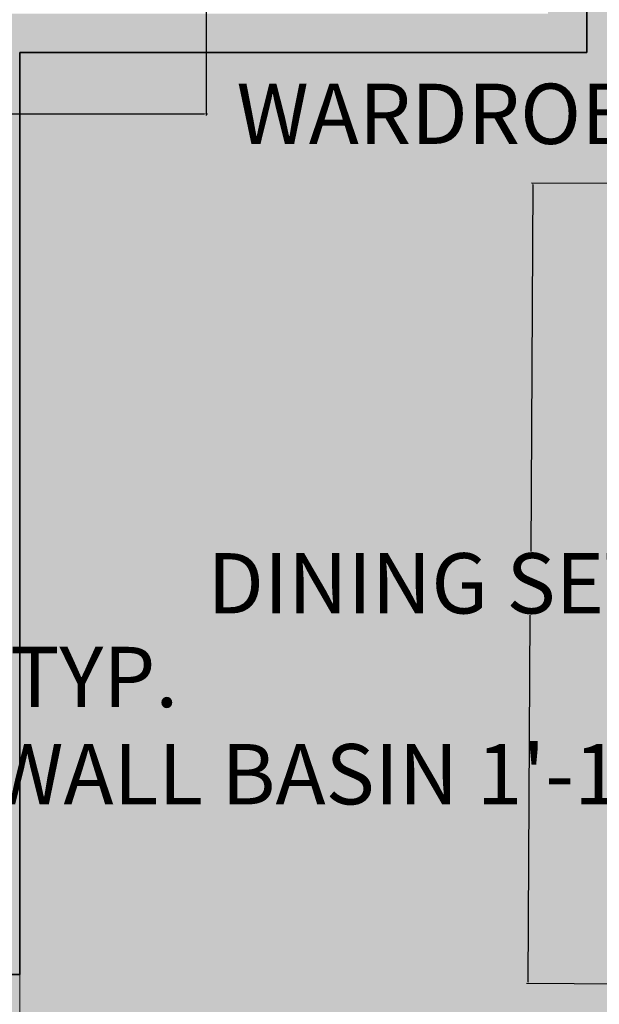
# Model space of a CAD drawing. Units: inches. Extents: x 1316 to 1777, y 813 to 1650.
# Tile 8 of 22: x 1445 to 1512, y 1319 to 1434. Entities that reach past the tile are written whole.
import ezdxf

# ---------------------------------------------------------------- set-up
doc = ezdxf.new("R2010")
doc.units = ezdxf.units.IN
doc.header["$MEASUREMENT"] = 0
doc.linetypes.add('ACAD_ISO02W100', pattern=[15, 12, -3])
for name, color, linetype, lineweight in [('A-ANNO-DIMS', 2, 'Continuous', 18), ('A-WALL-OVHD', 250, 'ACAD_ISO02W100', 18), ('A-WALL-PATT', 250, 'Continuous', 13), ('walls', 250, 'Continuous', 35)]:
    doc.layers.add(name, color=color, linetype=linetype, lineweight=lineweight)
doc.layers.add('A-FLOR-PATT', color=254, linetype='Continuous', lineweight=13, true_color=0xfeeab9)
doc.styles.get("Standard").update_dxf_attribs({"font": 'arial.ttf'})
doc.dimstyles.get("Standard").update_dxf_attribs({"dimtxt": 7, "dimasz": 0.18, "dimexe": 0.18, "dimexo": 0.0625, "dimgap": 0.09, "dimtad": 0, "dimtih": 1, "dimtoh": 1, "dimzin": 0, "dimdsep": 46, "dimlunit": 3, "dimtxsty": 'Standard', "dimcen": 0.09, "dimadec": 0, "dimazin": 0, "dimtfac": 1, "dimtofl": 0, "dimtmove": 0, "dimatfit": 3, "dimfxl": 1, "dimtolj": 1, "dimtzin": 0, "dimarcsym": 0})

# ---------------------------------------------------------------- blocks, each defined once
blk = doc.blocks.new('*D30')
at = {"layer": 'A-ANNO-DIMS', "color": 0, "lineweight": -2, "transparency": 16777216}
for p, q in [((1386.15, 1434.7), (1386.15, 1422.58)), ((1466.18, 1434.7), (1466.18, 1422.58)), ((1386.33, 1422.76), (1466, 1422.76)), ((1466.18, 1422.76), (1466.36, 1422.76))]:
    blk.add_line(p, q, dxfattribs=at)
at = {"layer": 'A-ANNO-DIMS', "color": 0, "transparency": 16777216}
for points in [[(1386.33, 1422.79), (1386.33, 1422.73), (1386.15, 1422.76)], [(1466, 1422.79), (1466, 1422.73), (1466.18, 1422.76)]]:
    blk.add_solid(points, dxfattribs=at)
at = {"layer": 'Defpoints', "color": 0, "transparency": 16777216}
for p in [(1386.15, 1434.76), (1466.18, 1434.76), (1466.18, 1422.76)]:
    blk.add_point(p, dxfattribs=at)
at = {"layer": 'A-ANNO-DIMS', "color": 0, "transparency": 16777216, "insert": (1518.08, 1422.76), "char_height": 7, "attachment_point": 5}
blk.add_mtext('\\A1;WARDROBE 6\'-8" TYP.', dxfattribs=at)
blk = doc.blocks.new('*D31')
at = {"layer": 'A-ANNO-DIMS', "color": 0, "lineweight": -2, "transparency": 16777216}
for p, q in [((1466.24, 1450.33), (1478.36, 1450.33)), ((1478.18, 1450.15), (1478.18, 1446.26)), ((1478.18, 1434.94), (1478.18, 1438.83)), ((1466.24, 1434.76), (1478.36, 1434.76))]:
    blk.add_line(p, q, dxfattribs=at)
at = {"layer": 'A-ANNO-DIMS', "color": 0, "transparency": 16777216}
for points in [[(1478.15, 1450.15), (1478.21, 1450.15), (1478.18, 1450.33)], [(1478.15, 1434.94), (1478.21, 1434.94), (1478.18, 1434.76)]]:
    blk.add_solid(points, dxfattribs=at)
at = {"layer": 'Defpoints', "color": 0, "transparency": 16777216}
for p in [(1466.18, 1450.33), (1478.18, 1450.33), (1466.18, 1434.76)]:
    blk.add_point(p, dxfattribs=at)
at = {"layer": 'A-ANNO-DIMS', "color": 0, "transparency": 16777216, "insert": (1478.18, 1442.55), "char_height": 7, "attachment_point": 5}
blk.add_mtext('\\A1;1\'-3 1/2" TYP.', dxfattribs=at)
blk = doc.blocks.new('*D36')
at = {"layer": 'A-ANNO-DIMS', "color": 0, "lineweight": -2, "transparency": 16777216}
for p, q in [((1416.11, 1349.39), (1416.11, 1345.95)), ((1438.26, 1349.39), (1438.26, 1345.95)), ((1416.29, 1346.13), (1438.08, 1346.13)), ((1438.26, 1346.13), (1438.44, 1346.13))]:
    blk.add_line(p, q, dxfattribs=at)
at = {"layer": 'A-ANNO-DIMS', "color": 0, "transparency": 16777216}
for points in [[(1416.29, 1346.16), (1416.29, 1346.1), (1416.11, 1346.13)], [(1438.08, 1346.16), (1438.08, 1346.1), (1438.26, 1346.13)]]:
    blk.add_solid(points, dxfattribs=at)
at = {"layer": 'Defpoints', "color": 0, "transparency": 16777216}
for p in [(1416.11, 1349.46), (1438.26, 1349.46), (1438.26, 1346.13)]:
    blk.add_point(p, dxfattribs=at)
at = {"layer": 'A-ANNO-DIMS', "color": 0, "transparency": 16777216, "insert": (1493.43, 1346.13), "char_height": 7, "attachment_point": 5}
blk.add_mtext('\\A1;WALL BASIN 1\'-10" TYP.', dxfattribs=at)
blk = doc.blocks.new('*D37')
at = {"layer": 'A-ANNO-DIMS', "color": 0, "lineweight": -2, "transparency": 16777216}
for p, q in [((1438.33, 1365.37), (1441.77, 1365.37)), ((1441.59, 1365.19), (1441.59, 1361.02)), ((1441.59, 1349.64), (1441.59, 1353.81)), ((1438.33, 1349.46), (1441.77, 1349.46))]:
    blk.add_line(p, q, dxfattribs=at)
at = {"layer": 'A-ANNO-DIMS', "color": 0, "transparency": 16777216}
for points in [[(1441.56, 1365.19), (1441.62, 1365.19), (1441.59, 1365.37)], [(1441.56, 1349.64), (1441.62, 1349.64), (1441.59, 1349.46)]]:
    blk.add_solid(points, dxfattribs=at)
at = {"layer": 'Defpoints', "color": 0, "transparency": 16777216}
for p in [(1438.26, 1365.37), (1441.59, 1365.37), (1438.26, 1349.46)]:
    blk.add_point(p, dxfattribs=at)
at = {"layer": 'A-ANNO-DIMS', "color": 0, "transparency": 16777216, "insert": (1441.59, 1357.41), "char_height": 7, "attachment_point": 5}
blk.add_mtext('\\A1;1\'-4" TYP.', dxfattribs=at)
blk = doc.blocks.new('*D40')
at = {"layer": 'A-ANNO-DIMS', "color": 0, "lineweight": -2, "transparency": 16777216}
for p, q in [((1388.84, 1302.16), (1388.84, 1312.14)), ((1389.02, 1311.96), (1454.4, 1311.96)), ((1454.58, 1302.16), (1454.58, 1312.14)), ((1454.58, 1311.96), (1454.76, 1311.96))]:
    blk.add_line(p, q, dxfattribs=at)
at = {"layer": 'A-ANNO-DIMS', "color": 0, "transparency": 16777216}
for points in [[(1389.02, 1311.99), (1389.02, 1311.93), (1388.84, 1311.96)], [(1454.4, 1311.99), (1454.4, 1311.93), (1454.58, 1311.96)]]:
    blk.add_solid(points, dxfattribs=at)
at = {"layer": 'Defpoints', "color": 0, "transparency": 16777216}
for p in [(1454.58, 1311.96), (1388.84, 1302.1), (1454.58, 1302.1)]:
    blk.add_point(p, dxfattribs=at)
at = {"layer": 'A-ANNO-DIMS', "color": 0, "transparency": 16777216, "insert": (1507.74, 1311.96), "char_height": 7, "attachment_point": 5}
blk.add_mtext('\\A1;KITCHEN SINK 5\'-5 1/2"', dxfattribs=at)
blk = doc.blocks.new('*D42')
at = {"layer": 'A-ANNO-DIMS', "color": 0, "lineweight": -2, "transparency": 16777216}
for p, q in [((1388.61, 1310.85), (1388.61, 1307.49)), ((1410.21, 1310.85), (1410.21, 1307.49)), ((1388.79, 1307.67), (1410.03, 1307.67)), ((1410.21, 1307.67), (1410.39, 1307.67))]:
    blk.add_line(p, q, dxfattribs=at)
at = {"layer": 'A-ANNO-DIMS', "color": 0, "transparency": 16777216}
for points in [[(1388.79, 1307.7), (1388.79, 1307.64), (1388.61, 1307.67)], [(1410.03, 1307.7), (1410.03, 1307.64), (1410.21, 1307.67)]]:
    blk.add_solid(points, dxfattribs=at)
at = {"layer": 'Defpoints', "color": 0, "transparency": 16777216}
for p in [(1388.61, 1310.91), (1410.21, 1310.91), (1410.21, 1307.67)]:
    blk.add_point(p, dxfattribs=at)
at = {"layer": 'A-ANNO-DIMS', "color": 0, "transparency": 16777216, "insert": (1453.71, 1307.67), "char_height": 7, "attachment_point": 5}
blk.add_mtext('\\A1;COOKTOP 1\'-9 1/2"', dxfattribs=at)
blk = doc.blocks.new('*D48')
at = {"layer": 'A-ANNO-DIMS', "color": 0, "lineweight": -2, "transparency": 16777216}
for p, q in [((1504.09, 1414.55), (1503.83, 1371.99)), ((1517.96, 1414.64), (1503.91, 1414.73)), ((1503.52, 1322.01), (1503.78, 1364.57)), ((1517.39, 1321.74), (1503.34, 1321.83))]:
    blk.add_line(p, q, dxfattribs=at)
at = {"layer": 'A-ANNO-DIMS', "color": 0, "transparency": 16777216}
for points in [[(1504.06, 1414.55), (1504.12, 1414.55), (1504.09, 1414.73)], [(1503.49, 1322.01), (1503.55, 1322.01), (1503.52, 1321.83)]]:
    blk.add_solid(points, dxfattribs=at)
at = {"layer": 'Defpoints', "color": 0, "transparency": 16777216}
for p in [(1518.02, 1414.64), (1503.52, 1321.83), (1517.46, 1321.74)]:
    blk.add_point(p, dxfattribs=at)
at = {"layer": 'A-ANNO-DIMS', "color": 0, "transparency": 16777216, "insert": (1503.81, 1368.28), "char_height": 7, "attachment_point": 5}
blk.add_mtext('\\A1;DINING SET 7\'-9"', dxfattribs=at)

msp = doc.modelspace()

# ---------------------------------------------------------------- hatches: boundary and pattern name
at = {"layer": 'A-FLOR-PATT'}
h = msp.add_hatch(color=256, dxfattribs=at)
h.dxf.hatch_style = 1
h.paths.add_polyline_path([(1567.673, 1281.369), (1651.673, 1281.369), (1651.673, 1365.369), (1597.673, 1365.369), (1597.673, 1429.869), (1570.345, 1429.869), (1570.345, 1471.869), (1510.345, 1471.869), (1510.345, 1429.869), (1444.564, 1429.869), (1444.564, 1322.882), (1444.564, 1300.088), (1510.564, 1300.088), (1510.564, 1295.094), (1510.564, 1240.869), (1386.064, 1240.869), (1386.064, 1171.185), (1400.961, 1171.185), (1400.961, 1106.742), (1386.064, 1106.742), (1386.064, 1072.869), (1510.564, 1072.869), (1510.564, 1040.173), (1541.068, 1040.173, -0.367085), (1572.764, 1069.547), (1572.764, 1069.579), (1574.225, 1069.579), (1574.225, 1040.173), (1616.037, 1040.173), (1616.037, 1086.627), (1616.037, 1103.705), (1613.066, 1105.235), (1616.037, 1106.686), (1616.037, 1123.869), (1567.673, 1123.869)])
h.paths.add_polyline_path([(1508.987, 1198.018), (1511.117, 1198.018), (1511.117, 1200.148), (1532.595, 1200.148), (1532.595, 1198.018), (1534.725, 1198.018), (1534.725, 1176.008), (1530.465, 1176.008), (1530.465, 1176.718), (1513.247, 1176.718), (1513.247, 1176.008), (1508.987, 1176.008)], flags=16)
h.paths.add_polyline_path([(1505.979, 1151.315), (1521.504, 1151.315), (1521.504, 1123.623), (1505.979, 1123.623)], flags=16)
h.paths.add_polyline_path([(1507.734, 1150.101, -1), (1506.932, 1150.101, -1)], flags=0)
h.paths.add_polyline_path([(1512.288, 1138.353), (1512.28, 1138.392), (1512.219, 1138.376)], flags=0)
h.paths.add_polyline_path([(1511.539, 1138.926), (1511.802, 1138.967), (1511.817, 1139.27), (1511.607, 1139.246)], flags=0)
h.paths.add_polyline_path([(1513.745, 1140.234), (1513.68, 1139.885), (1514.014, 1140.045), (1513.855, 1140.308)], flags=0)
h.paths.add_polyline_path([(1513.759, 1139.089), (1514.005, 1139.255), (1513.807, 1139.483), (1513.564, 1139.327)], flags=0)
h.paths.add_polyline_path([(1514.219, 1138.385), (1514.336, 1138.33), (1514.544, 1138.32), (1514.802, 1138.874), (1514.451, 1138.716)], flags=0)
h.paths.add_polyline_path([(1514.577, 1137.439), (1514.573, 1137.4), (1514.699, 1137.4), (1514.696, 1137.402)], flags=0)
h.paths.add_polyline_path([(1512.26, 1136.199), (1512.199, 1136.399), (1512.032, 1136.325), (1512.095, 1136.101), (1512.257, 1136.192)], flags=0)
h.paths.add_polyline_path([(1512.644, 1137.274), (1512.356, 1137.23), (1512.432, 1137.049), (1512.703, 1137.093)], flags=0)
h.paths.add_polyline_path([(1513.049, 1137.593), (1512.979, 1137.8), (1512.843, 1137.757), (1512.887, 1137.556)], flags=0)
h.paths.add_polyline_path([(1513.269, 1138.556), (1513.571, 1137.962), (1513.459, 1136.814), (1513.212, 1137.878), (1513.032, 1138.443)], flags=0)
h.paths.add_polyline_path([(1514.891, 1136.377), (1514.696, 1136.401), (1514.683, 1136.246), (1514.87, 1136.165)], flags=0)
h.paths.add_polyline_path([(1514.142, 1137.293), (1514.047, 1136.743), (1514.27, 1136.751), (1514.328, 1137.265)], flags=0)
h.paths.add_polyline_path([(1515.362, 1138.976), (1515.334, 1138.638), (1515.596, 1138.588), (1515.627, 1138.932)], flags=0)
h.paths.add_polyline_path([(1537.285, 1177.912), (1537.995, 1177.912), (1537.995, 1195.13), (1537.285, 1195.13), (1537.285, 1199.39), (1559.295, 1199.39), (1559.295, 1197.26), (1561.425, 1197.26), (1561.425, 1175.782), (1559.295, 1175.782), (1559.295, 1173.652), (1559.379, 1173.652), (1559.379, 1171.514), (1561.517, 1171.514), (1561.517, 1098.819), (1559.379, 1098.819), (1559.379, 1096.68), (1537.285, 1096.68), (1537.285, 1100.957), (1537.997, 1100.957), (1537.997, 1169.376), (1537.285, 1169.376), (1537.285, 1173.652)], flags=16)
h.paths.add_polyline_path([(1518.623, 1345.565), (1519.133, 1345.48), (1519.133, 1345.485), (1518.623, 1345.567)], flags=16)
h.paths.add_polyline_path([(1518.798, 1374.15), (1519.308, 1374.064), (1519.308, 1374.069), (1518.798, 1374.152)], flags=16)
h.paths.add_polyline_path([(1537.764, 1413.501), (1537.678, 1412.991), (1537.683, 1412.991), (1537.766, 1413.501)], flags=16)
h.paths.add_polyline_path([(1572.905, 1373.821), (1573.927, 1373.975), (1574.027, 1390.309), (1573.007, 1390.475), (1573.007, 1390.475)], flags=16)
h.paths.add_polyline_path([(1572.73, 1345.237), (1573.752, 1345.39), (1573.852, 1361.724), (1572.832, 1361.89), (1572.832, 1361.89)], flags=16)
h.paths.add_polyline_path([(1537.211, 1322.643), (1537.364, 1321.621), (1553.698, 1321.521), (1553.864, 1322.541)], flags=16)
h.paths.add_polyline_path([(1535.908, 1331.328), (1527.214, 1331.382), (1527.664, 1404.885), (1564.416, 1404.66), (1563.966, 1331.157), (1555.273, 1331.21), (1553.947, 1323.051), (1537.134, 1323.154)], flags=16)
h.paths.add_polyline_path([(1536.15, 1336.503), (1536.235, 1337.572), (1536.323, 1338.628), (1536.411, 1339.663), (1536.495, 1340.67), (1536.574, 1341.66), (1536.648, 1342.648), (1536.717, 1343.649), (1536.78, 1344.678), (1536.837, 1345.75), (1536.913, 1347.475), (1536.93, 1348.082), (1536.867, 1346.314), (1536.754, 1344.188), (1536.619, 1342.219), (1536.495, 1340.67), (1536.411, 1339.663), (1536.323, 1338.628), (1536.235, 1337.572), (1536.15, 1336.503), (1536.071, 1335.432), (1536.002, 1334.37), (1535.917, 1332.754), (1535.909, 1332.308), (1535.964, 1333.78), (1536.071, 1335.432)], flags=0)
h.paths.add_polyline_path([(1540.412, 1338.345), (1540.539, 1339.037), (1540.667, 1339.758), (1540.798, 1340.518), (1540.93, 1341.325), (1541.063, 1342.187), (1541.196, 1343.109), (1541.326, 1344.085), (1541.45, 1345.102), (1541.566, 1346.15), (1541.669, 1347.219), (1541.758, 1348.296), (1541.829, 1349.371), (1541.879, 1350.434), (1541.906, 1351.476), (1541.91, 1352.5), (1541.895, 1353.512), (1541.861, 1354.518), (1541.812, 1355.524), (1541.749, 1356.537), (1541.674, 1357.561), (1541.551, 1359.062), (1541.495, 1359.67), (1541.589, 1358.603), (1541.721, 1356.977), (1541.846, 1354.98), (1541.912, 1352.982), (1541.903, 1350.951), (1541.806, 1348.87), (1541.628, 1346.713), (1541.396, 1344.612), (1541.135, 1342.656), (1540.872, 1340.947), (1540.617, 1339.466), (1540.412, 1338.345), (1540.288, 1337.675), (1540.166, 1337.018), (1540.049, 1336.365), (1539.937, 1335.71), (1539.837, 1335.055), (1539.758, 1334.403), (1539.709, 1333.756), (1539.697, 1333.12), (1539.751, 1332.162), (1539.822, 1331.89), (1539.691, 1332.775), (1539.714, 1334.035), (1539.867, 1335.303), (1540.085, 1336.577), (1540.288, 1337.675)], flags=0)
h.paths.add_polyline_path([(1545.599, 1331.584), (1545.601, 1331.617), (1545.614, 1331.689), (1545.737, 1332.197), (1545.767, 1332.332), (1545.84, 1332.681), (1545.925, 1333.114), (1546.016, 1333.614), (1546.108, 1334.164), (1546.196, 1334.748), (1546.276, 1335.349), (1546.342, 1335.952), (1546.388, 1336.539), (1546.412, 1337.098), (1546.414, 1337.632), (1546.395, 1338.145), (1546.359, 1338.645), (1546.306, 1339.137), (1546.24, 1339.627), (1546.161, 1340.121), (1546.073, 1340.625), (1545.888, 1341.63), (1545.718, 1342.621), (1545.547, 1343.945), (1545.432, 1345.534), (1545.404, 1347.402), (1545.418, 1348.013), (1545.411, 1346.957), (1545.425, 1345.988), (1545.463, 1345.105), (1545.521, 1344.301), (1545.596, 1343.566), (1545.683, 1342.892), (1545.778, 1342.27), (1545.877, 1341.691), (1545.977, 1341.145), (1546.133, 1340.297), (1546.327, 1339.075), (1546.434, 1337.615), (1546.377, 1336.279), (1546.246, 1335.079), (1546.032, 1333.665), (1545.84, 1332.681), (1545.767, 1332.332)], flags=0)
h.paths.add_polyline_path([(1551.803, 1337.656), (1551.963, 1338.25), (1552.102, 1338.801), (1552.225, 1339.338), (1552.331, 1339.865), (1552.418, 1340.377), (1552.487, 1340.873), (1552.536, 1341.348), (1552.563, 1341.801), (1552.569, 1342.228), (1552.551, 1342.627), (1552.51, 1342.995), (1552.446, 1343.333), (1552.363, 1343.646), (1552.261, 1343.937), (1552.144, 1344.207), (1552.012, 1344.461), (1551.868, 1344.7), (1551.746, 1344.882), (1550.887, 1346.052), (1550.428, 1347.126), (1550.183, 1348.353), (1550.048, 1349.632), (1549.978, 1351.224), (1549.974, 1353.141), (1549.989, 1353.748), (1549.975, 1352.682), (1549.977, 1351.708), (1549.996, 1350.825), (1550.031, 1350.027), (1550.082, 1349.31), (1550.15, 1348.669), (1550.234, 1348.098), (1550.335, 1347.593), (1550.452, 1347.149), (1550.584, 1346.76), (1550.73, 1346.419), (1550.887, 1346.117), (1551.05, 1345.848), (1551.217, 1345.602), (1551.386, 1345.372), (1551.553, 1345.151), (1552, 1344.537), (1552.454, 1343.495), (1552.591, 1342.266), (1552.509, 1340.905), (1552.246, 1339.367), (1551.925, 1338.101), (1551.619, 1336.984), (1551.406, 1336.2), (1551.01, 1334.699), (1550.877, 1334.155), (1551.264, 1335.677), (1551.619, 1336.984)], flags=0)
h.paths.add_polyline_path([(1558.642, 1348.348), (1558.795, 1348.811), (1558.918, 1349.215), (1559.008, 1349.575), (1559.061, 1349.904), (1559.076, 1350.214), (1559.054, 1350.506), (1559.001, 1350.776), (1558.919, 1351.021), (1558.814, 1351.239), (1558.688, 1351.425), (1558.546, 1351.578), (1558.392, 1351.694), (1558.229, 1351.772), (1558.059, 1351.812), (1557.882, 1351.819), (1557.701, 1351.794), (1557.515, 1351.742), (1557.327, 1351.665), (1557.136, 1351.566), (1556.944, 1351.448), (1556.752, 1351.315), (1556.742, 1351.307), (1556.175, 1350.878), (1555.982, 1350.741), (1555.79, 1350.618), (1555.103, 1350.248), (1554.019, 1350.696), (1553.658, 1351.734), (1553.592, 1352.861), (1553.705, 1354.248), (1553.753, 1354.657), (1553.685, 1354.004), (1553.638, 1353.425), (1553.615, 1352.918), (1553.615, 1352.476), (1553.637, 1352.094), (1553.681, 1351.766), (1553.745, 1351.485), (1553.828, 1351.246), (1553.929, 1351.043), (1554.048, 1350.87), (1554.182, 1350.722), (1554.33, 1350.599), (1554.491, 1350.501), (1554.662, 1350.43), (1554.841, 1350.388), (1555.026, 1350.374), (1555.215, 1350.39), (1555.406, 1350.437), (1555.598, 1350.514), (1555.79, 1350.618), (1555.982, 1350.741), (1556.175, 1350.878), (1556.367, 1351.024), (1556.559, 1351.171), (1556.752, 1351.315), (1556.944, 1351.448), (1557.136, 1351.566), (1557.327, 1351.665), (1558.043, 1351.957), (1558.894, 1351.316), (1559.137, 1350.09), (1558.886, 1349.087), (1558.642, 1348.348), (1558.463, 1347.812), (1558.261, 1347.187), (1558.039, 1346.459), (1557.677, 1345.175), (1557.549, 1344.636), (1557.909, 1346.03), (1558.329, 1347.408)], flags=0)
h.paths.add_polyline_path([(1562.145, 1353.919), (1562.25, 1354.68), (1562.341, 1355.344), (1562.416, 1355.924), (1562.475, 1356.431), (1562.518, 1356.872), (1562.544, 1357.254), (1562.554, 1357.582), (1562.548, 1357.862), (1562.525, 1358.1), (1562.486, 1358.303), (1562.432, 1358.476), (1562.361, 1358.624), (1562.277, 1358.748), (1562.18, 1358.848), (1562.073, 1358.925), (1561.958, 1358.977), (1561.837, 1359.006), (1561.711, 1359.011), (1561.584, 1358.992), (1561.456, 1358.949), (1561.342, 1358.895), (1560.78, 1358.554), (1560.631, 1358.473), (1560.474, 1358.403), (1560.311, 1358.348), (1559.637, 1358.207), (1558.973, 1358.904), (1558.816, 1360.002), (1558.804, 1361.236), (1558.83, 1361.674), (1558.807, 1360.917), (1558.813, 1360.297), (1558.845, 1359.795), (1558.902, 1359.397), (1558.982, 1359.087), (1559.082, 1358.849), (1559.2, 1358.666), (1559.334, 1358.525), (1559.482, 1358.421), (1559.639, 1358.351), (1559.804, 1358.311), (1559.973, 1358.3), (1560.143, 1358.313), (1560.311, 1358.348), (1560.474, 1358.403), (1560.631, 1358.473), (1560.78, 1358.554), (1560.923, 1358.641), (1561.061, 1358.729), (1561.196, 1358.813), (1561.382, 1358.92), (1561.342, 1358.895), (1561.972, 1359.194), (1562.536, 1358.367), (1562.56, 1357.311), (1562.455, 1356.226), (1562.323, 1355.206), (1562.145, 1353.919), (1562.026, 1353.049), (1561.815, 1351.457), (1561.752, 1350.933), (1561.948, 1352.479)], flags=0)
h.paths.add_polyline_path([(1572.764, 1069.547, 0.367085), (1541.068, 1040.173), (1572.764, 1040.173)], flags=17)
h.paths.add_polyline_path([(1572.764, 1040.173), (1541.068, 1040.173, 0.0299535), (1540.829, 1036.182), (1540.829, 1031.173), (1574.225, 1031.173), (1574.225, 1036.182), (1572.764, 1036.182)])
h = msp.add_hatch(color=256, dxfattribs=at)
h.dxf.hatch_style = 1
h.paths.add_polyline_path([(1440.064, 1429.869), (1386.064, 1429.869), (1386.064, 1369.869), (1440.064, 1369.869), (1440.064, 1372.189), (1411.168, 1372.189), (1411.168, 1373.459), (1411.196, 1373.459, -0.4000145), (1440.064, 1401.229)])
h.paths.add_polyline_path([(1444.564, 1401.229), (1440.208, 1401.229, 0.4014527), (1411.196, 1373.459), (1440.208, 1373.459), (1440.208, 1372.189), (1444.564, 1372.189)])
h = msp.add_hatch(color=256, dxfattribs=at)
h.dxf.hatch_style = 1
h.paths.add_polyline_path([(1506.064, 1295.094), (1444.564, 1295.094), (1444.564, 1322.882), (1440.064, 1322.882), (1440.064, 1346.929), (1412.858, 1346.929), (1412.858, 1245.369), (1506.064, 1245.369)])
h.paths.add_polyline_path([(1484.665, 1269.305), (1504.59, 1269.305), (1504.59, 1245.841), (1484.665, 1245.841)], flags=16)
h.paths.add_polyline_path([(1510.564, 1300.088), (1444.564, 1300.088), (1444.564, 1295.094), (1506.064, 1295.094), (1510.564, 1295.094)])
at = {"layer": 'A-WALL-PATT'}
h = msp.add_hatch(color=256, dxfattribs=at)
h.dxf.hatch_style = 1
h.paths.add_polyline_path([(1713.173, 1281.369), (1656.173, 1281.369), (1656.173, 1298.258), (1651.673, 1298.258), (1651.673, 1281.369), (1567.673, 1281.369), (1567.673, 1266.995), (1572.173, 1266.995), (1572.173, 1276.869), (1704.173, 1276.869), (1704.173, 1132.869), (1608.64, 1132.869), (1608.64, 1123.869), (1704.173, 1123.869), (1704.173, 1040.173), (1652.869, 1040.173), (1652.869, 1031.173), (1713.173, 1031.173), (1713.173, 1040.173)])
h.paths.add_polyline_path([(1572.173, 1237.955), (1567.673, 1237.955), (1567.673, 1123.869), (1583.146, 1123.869), (1583.146, 1132.869), (1572.173, 1132.869)], flags=17)
h.paths.add_polyline_path([(1510.345, 1566.369), (1524.171, 1566.369), (1524.171, 1571.985), (1524.171, 1575.369), (1445.955, 1575.369), (1445.955, 1566.369), (1505.845, 1566.369), (1505.845, 1469.591), (1510.345, 1469.591), (1510.345, 1471.869), (1529.081, 1471.869), (1529.081, 1476.369), (1510.345, 1476.369)])
h.paths.add_polyline_path([(1609.722, 1575.369), (1545.119, 1575.369), (1545.119, 1566.369), (1570.345, 1566.369), (1570.345, 1476.369), (1562.477, 1476.369), (1562.477, 1471.869), (1570.345, 1471.869), (1570.345, 1469.591), (1574.845, 1469.591), (1574.845, 1566.369), (1609.722, 1566.369)])
h.paths.add_polyline_path([(1713.173, 1575.369), (1655.233, 1575.369), (1655.233, 1566.369), (1704.173, 1566.369), (1704.173, 1434.369), (1574.845, 1434.369), (1574.845, 1440.551), (1574.701, 1440.551), (1570.345, 1440.551), (1570.345, 1429.869), (1597.673, 1429.869), (1597.673, 1408.281), (1602.173, 1408.281), (1602.173, 1429.869), (1704.173, 1429.869), (1704.173, 1410.704), (1707.375, 1410.704), (1713.173, 1410.704)])
h.paths.add_polyline_path([(1713.173, 1383.676), (1704.173, 1383.676), (1704.173, 1369.869), (1602.173, 1369.869), (1602.173, 1379.241), (1597.673, 1379.241), (1597.673, 1365.369), (1713.173, 1365.369)])
h.paths.add_polyline_path([(1444.564, 1429.869), (1510.345, 1429.869), (1510.345, 1440.551), (1505.845, 1440.551), (1505.845, 1434.369), (1386.064, 1434.369), (1386.064, 1566.369), (1400.445, 1566.369), (1400.445, 1575.369), (1377.064, 1575.369), (1377.064, 1412.813), (1380.509, 1412.813), (1386.064, 1412.813), (1386.064, 1429.869), (1440.064, 1429.869), (1440.064, 1401.229), (1444.564, 1401.229)])
h.paths.add_polyline_path([(1444.564, 1372.189), (1440.064, 1372.189), (1440.064, 1369.869), (1386.064, 1369.869), (1386.064, 1378.758), (1377.064, 1378.758), (1377.064, 1349.201), (1381.118, 1349.201), (1386.064, 1349.201), (1386.064, 1365.369), (1440.064, 1365.369), (1440.064, 1322.882), (1444.564, 1322.882)])
h.paths.add_polyline_path([(1510.564, 1295.094), (1506.064, 1295.094), (1506.064, 1245.369), (1386.064, 1245.369), (1386.064, 1272.582), (1377.064, 1272.582), (1377.064, 1212.905), (1380.1, 1212.905), (1386.064, 1212.905), (1386.064, 1240.869), (1510.564, 1240.869)])
h.paths.add_polyline_path([(1386.064, 1163.761), (1377.064, 1163.761), (1377.064, 1063.869), (1419.363, 1063.869), (1419.363, 1072.869), (1386.064, 1072.869)])
h.paths.add_polyline_path([(1510.564, 1072.869), (1469.381, 1072.869), (1469.381, 1063.869), (1501.564, 1063.869), (1501.564, 1033.023), (1501.564, 1031.173), (1540.829, 1031.173), (1540.829, 1036.182, -0.0299535), (1541.068, 1040.173), (1510.564, 1040.173)])
h.paths.add_polyline_path([(1607.369, 1040.173), (1574.225, 1040.173), (1574.225, 1036.182), (1574.225, 1031.173), (1607.369, 1031.173)], flags=17)
h.paths.add_polyline_path([(1637.054, 1040.173), (1624.706, 1040.173), (1624.706, 1031.173), (1637.054, 1031.173)], flags=17)

# ---------------------------------------------------------------- linework, layer by layer
at = {"layer": 'A-WALL-OVHD'}
msp.add_line((1444.564, 1322.882), (1444.564, 1295.189), dxfattribs=at)
at = {"layer": 'walls'}
for p, q in [((1510.345, 1471.869), (1510.345, 1429.869)), ((1444.564, 1429.869), (1444.564, 1322.882)), ((1444.564, 1429.869), (1510.345, 1429.869)), ((1440.064, 1322.882), (1444.564, 1322.882))]:
    msp.add_line(p, q, dxfattribs=at)

# ---------------------------------------------------------------- dimensions: what is measured, and where the dimension line sits
at = {"layer": 'A-ANNO-DIMS'}
for base, p1, p2, angle, text, picture, middle in [((1478.181, 1450.329), (1466.177, 1434.762), (1466.177, 1450.329), 90, '<> TYP.', '*D31', (1478.181, 1442.545)), ((1503.522, 1321.828), (1518.025, 1414.643), (1517.457, 1321.742), 269.6497, 'DINING SET <>', '*D48', (1503.806, 1368.278)), ((1441.586, 1365.369), (1438.263, 1349.455), (1438.263, 1365.369), 90, '<> TYP.', '*D37', (1441.586, 1357.412))]:
    dim = msp.add_linear_dim(base=base, p1=p1, p2=p2, angle=angle, text=text, dimstyle='Standard', override={"dimdec": 1, "dimlfac": 1, "dimrnd": 0, "dimzin": 1, "dimdsep": 46, "dimlunit": 4, "dimfrac": 2}, dxfattribs=at)
    dim.commit()
    dim.dimension.update_dxf_attribs({"geometry": picture, "text_midpoint": middle})
for base, p1, p2, text, picture, middle in [((1466.177, 1422.758), (1386.153, 1434.762), (1466.177, 1434.762), 'WARDROBE <> TYP.', '*D30', (1518.078, 1422.758)), ((1438.263, 1346.132), (1416.108, 1349.455), (1438.263, 1349.455), 'WALL BASIN <> TYP.', '*D36', (1493.435, 1346.132)), ((1454.577, 1311.961), (1388.838, 1302.1), (1454.577, 1302.1), 'KITCHEN SINK <>', '*D40', (1507.741, 1311.961)), ((1410.21, 1307.675), (1388.61, 1310.915), (1410.21, 1310.915), 'COOKTOP <>', '*D42', (1453.708, 1307.675))]:
    dim = msp.add_linear_dim(base=base, p1=p1, p2=p2, text=text, dimstyle='Standard', override={"dimdec": 1, "dimlfac": 1, "dimrnd": 0, "dimzin": 1, "dimdsep": 46, "dimlunit": 4, "dimfrac": 2}, dxfattribs=at)
    dim.commit()
    dim.dimension.update_dxf_attribs({"geometry": picture, "text_midpoint": middle})

doc.saveas('drawing.dxf')
